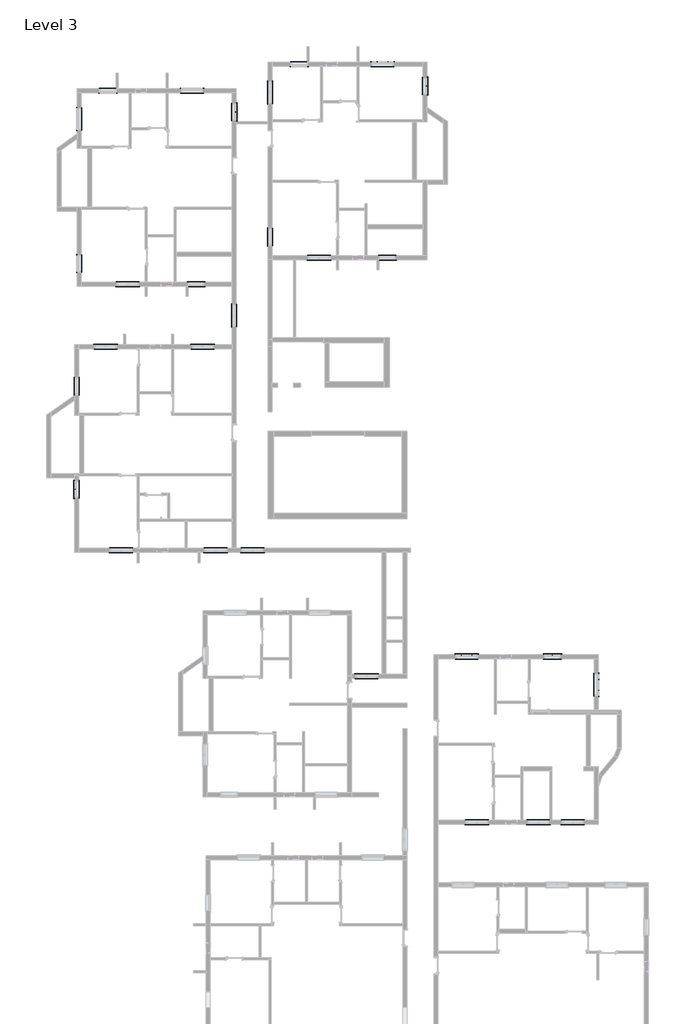
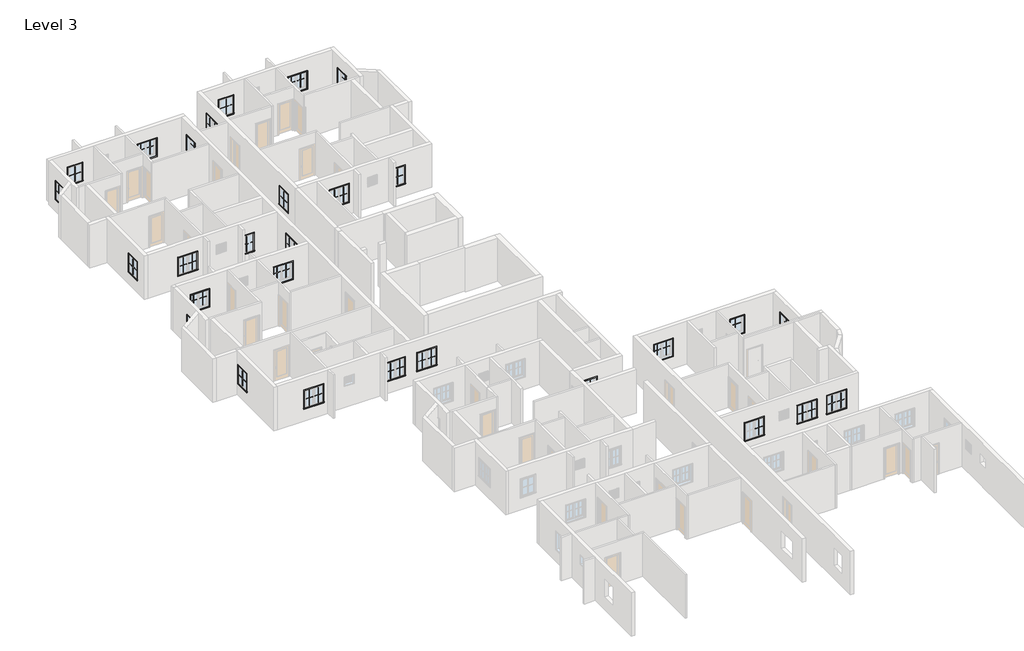
# One storey, part 7 of 7: 104 proxies.
"""IFC4 building model written with IfcOpenShell, lengths in millimetres."""

from ifc_helpers import new_model, si_unit, origin, place, context, project, spatial, transform, mapped, element, save
from components import muntin_pattern_2x2_muntin_pattern_2x2_95b57395, muntin_pattern_2x2_muntin_pattern_2x2_4dfeb3f3, muntin_pattern_2x2_muntin_pattern_2x2_e852a7e4, trim_window_exterior_flat_with_sill_e4b28ec3, trim_window_exterior_flat_with_sill_7cfdd449, trim_window_interior_flat_picture_frame_39ff4276, trim_window_interior_flat_picture_frame_f1e0b15b

model = new_model("IFC4")

# Units and contexts
model_context = context("Model", 3, world=origin())
ifc_project = project(units=[si_unit("LENGTHUNIT", "METRE", prefix="MILLI")], contexts=[model_context])

# Site, building, storey
site = spatial("IfcSite", under=ifc_project)
building = spatial("IfcBuilding", under=site)
storey = spatial("IfcBuildingStorey", under=building, Name="Level 3", Elevation=3200.4)

# Proxies
placement = place(None, origin())
muntin_pattern_2x2_muntin_pattern_2x2_shape = muntin_pattern_2x2_muntin_pattern_2x2_95b57395(model_context)
element("IfcBuildingElementProxy", 1, Name="Muntin Pattern_2x2 : Muntin Pattern_2x2", ObjectType="Muntin Pattern_2x2 : Muntin Pattern_2x2", at=placement, inside=storey, context=model_context, shape_type="MappedRepresentation", body=[
    mapped(muntin_pattern_2x2_muntin_pattern_2x2_shape, transform((-14884.6759469, 4921.5461172, 4184.65), x_axis=(0.0, 1.0, 0.0), y_axis=(-1.0, 0.0, 0.0), z_axis=(0.0, 0.0, 1.0))),
])
element("IfcBuildingElementProxy", 2, Name="Muntin Pattern_2x2 : Muntin Pattern_2x2", ObjectType="Muntin Pattern_2x2 : Muntin Pattern_2x2", at=placement, inside=storey, context=model_context, shape_type="MappedRepresentation", body=[
    mapped(muntin_pattern_2x2_muntin_pattern_2x2_shape, transform((-12990.7362554, 27537.0711172, 4184.65), x_axis=(-1.0, 0.0, 0.0), y_axis=(0.0, -1.0, 0.0), z_axis=(0.0, 0.0, 1.0))),
])
element("IfcBuildingElementProxy", 3, Name="Muntin Pattern_2x2 : Muntin Pattern_2x2", ObjectType="Muntin Pattern_2x2 : Muntin Pattern_2x2", at=placement, inside=storey, context=model_context, shape_type="MappedRepresentation", body=[
    mapped(muntin_pattern_2x2_muntin_pattern_2x2_shape, transform((-5683.5259469, 26431.1755084, 4184.65), x_axis=(0.0, -1.0, 0.0), y_axis=(1.0, 0.0, 0.0), z_axis=(0.0, 0.0, 1.0))),
])
element("IfcBuildingElementProxy", 4, Name="Muntin Pattern_2x2 : Muntin Pattern_2x2", ObjectType="Muntin Pattern_2x2 : Muntin Pattern_2x2", at=placement, inside=storey, context=model_context, shape_type="MappedRepresentation", body=[
    mapped(muntin_pattern_2x2_muntin_pattern_2x2_shape, transform((-7960.0009469, 16513.4711172, 4184.65), x_axis=(-1.0, 0.0, 0.0), y_axis=(0.0, -1.0, 0.0), z_axis=(0.0, 0.0, 1.0))),
])
element("IfcBuildingElementProxy", 5, Name="Muntin Pattern_2x2 : Muntin Pattern_2x2", ObjectType="Muntin Pattern_2x2 : Muntin Pattern_2x2", at=placement, inside=storey, context=model_context, shape_type="MappedRepresentation", body=[
    mapped(muntin_pattern_2x2_muntin_pattern_2x2_shape, transform((-14732.2759469, 17786.6461172, 4184.65), x_axis=(0.0, 1.0, 0.0), y_axis=(-1.0, 0.0, 0.0), z_axis=(0.0, 0.0, 1.0))),
])
element("IfcBuildingElementProxy", 6, Name="Muntin Pattern_2x2 : Muntin Pattern_2x2", ObjectType="Muntin Pattern_2x2 : Muntin Pattern_2x2", at=placement, inside=storey, context=model_context, shape_type="MappedRepresentation", body=[
    mapped(muntin_pattern_2x2_muntin_pattern_2x2_shape, transform((-2075.0862554, 29050.5505084, 4184.65), x_axis=(-1.0, 0.0, 0.0), y_axis=(0.0, -1.0, 0.0), z_axis=(0.0, 0.0, 1.0))),
])
element("IfcBuildingElementProxy", 7, Name="Muntin Pattern_2x2 : Muntin Pattern_2x2", ObjectType="Muntin Pattern_2x2 : Muntin Pattern_2x2", at=placement, inside=storey, context=model_context, shape_type="MappedRepresentation", body=[
    mapped(muntin_pattern_2x2_muntin_pattern_2x2_shape, transform((5213.0740531, 27910.7255084, 4184.65), x_axis=(0.0, -1.0, 0.0), y_axis=(1.0, 0.0, 0.0), z_axis=(0.0, 0.0, 1.0))),
])
element("IfcBuildingElementProxy", 8, Name="Muntin Pattern_2x2 : Muntin Pattern_2x2", ObjectType="Muntin Pattern_2x2 : Muntin Pattern_2x2", at=placement, inside=storey, context=model_context, shape_type="MappedRepresentation", body=[
    mapped(muntin_pattern_2x2_muntin_pattern_2x2_shape, transform((2936.5990531, 18026.9505084, 4184.65), x_axis=(-1.0, 0.0, 0.0), y_axis=(0.0, -1.0, 0.0), z_axis=(0.0, 0.0, 1.0))),
])
element("IfcBuildingElementProxy", 9, Name="Muntin Pattern_2x2 : Muntin Pattern_2x2", ObjectType="Muntin Pattern_2x2 : Muntin Pattern_2x2", at=placement, inside=storey, context=model_context, shape_type="MappedRepresentation", body=[
    mapped(muntin_pattern_2x2_muntin_pattern_2x2_shape, transform((-3835.6759469, 19300.1255084, 4184.65), x_axis=(0.0, 1.0, 0.0), y_axis=(-1.0, 0.0, 0.0), z_axis=(0.0, 0.0, 1.0))),
])
element("IfcBuildingElementProxy", 10, Name="Muntin Pattern_2x2 : Muntin Pattern_2x2", ObjectType="Muntin Pattern_2x2 : Muntin Pattern_2x2", at=placement, inside=storey, context=model_context, shape_type="MappedRepresentation", body=[
    mapped(muntin_pattern_2x2_muntin_pattern_2x2_shape, transform((12366.3490531, -4512.6747229, 4184.65), x_axis=(1.0, 0.0, 0.0), y_axis=(0.0, 1.0, 0.0), z_axis=(0.0, 0.0, 1.0))),
])
element("IfcBuildingElementProxy", 11, Name="Muntin Pattern_2x2 : Muntin Pattern_2x2", ObjectType="Muntin Pattern_2x2 : Muntin Pattern_2x2", at=placement, inside=storey, context=model_context, shape_type="MappedRepresentation", body=[
    mapped(muntin_pattern_2x2_muntin_pattern_2x2_shape, transform((-14675.1259469, 10795.2961172, 4184.65), x_axis=(0.0, -1.0, 0.0), y_axis=(1.0, 0.0, 0.0), z_axis=(0.0, 0.0, 1.0))),
])
muntin_pattern_2x2_muntin_pattern_2x2_2_shape = muntin_pattern_2x2_muntin_pattern_2x2_4dfeb3f3(model_context)
element("IfcBuildingElementProxy", 12, Name="Muntin Pattern_2x2 : Muntin Pattern_2x2", ObjectType="Muntin Pattern_2x2 : Muntin Pattern_2x2", at=placement, inside=storey, context=model_context, shape_type="MappedRepresentation", body=[
    mapped(muntin_pattern_2x2_muntin_pattern_2x2_2_shape, transform((-8498.1634469, 27746.6211172, 4184.65), x_axis=(1.0, 0.0, 0.0), y_axis=(0.0, 1.0, 0.0), z_axis=(0.0, 0.0, 1.0))),
])
element("IfcBuildingElementProxy", 13, Name="Muntin Pattern_2x2 : Muntin Pattern_2x2", ObjectType="Muntin Pattern_2x2 : Muntin Pattern_2x2", at=placement, inside=storey, context=model_context, shape_type="MappedRepresentation", body=[
    mapped(muntin_pattern_2x2_muntin_pattern_2x2_2_shape, transform((-14732.2759469, 25728.9086172, 4184.65), x_axis=(0.0, 1.0, 0.0), y_axis=(-1.0, 0.0, 0.0), z_axis=(0.0, 0.0, 1.0))),
])
element("IfcBuildingElementProxy", 14, Name="Muntin Pattern_2x2 : Muntin Pattern_2x2", ObjectType="Muntin Pattern_2x2 : Muntin Pattern_2x2", at=placement, inside=storey, context=model_context, shape_type="MappedRepresentation", body=[
    mapped(muntin_pattern_2x2_muntin_pattern_2x2_2_shape, transform((-11562.0384469, 16513.4711172, 4184.65), x_axis=(-1.0, 0.0, 0.0), y_axis=(0.0, -1.0, 0.0), z_axis=(0.0, 0.0, 1.0))),
])
element("IfcBuildingElementProxy", 15, Name="Muntin Pattern_2x2 : Muntin Pattern_2x2", ObjectType="Muntin Pattern_2x2 : Muntin Pattern_2x2", at=placement, inside=storey, context=model_context, shape_type="MappedRepresentation", body=[
    mapped(muntin_pattern_2x2_muntin_pattern_2x2_2_shape, transform((-3835.6759469, 27242.3880084, 4184.65), x_axis=(0.0, 1.0, 0.0), y_axis=(-1.0, 0.0, 0.0), z_axis=(0.0, 0.0, 1.0))),
])
element("IfcBuildingElementProxy", 16, Name="Muntin Pattern_2x2 : Muntin Pattern_2x2", ObjectType="Muntin Pattern_2x2 : Muntin Pattern_2x2", at=placement, inside=storey, context=model_context, shape_type="MappedRepresentation", body=[
    mapped(muntin_pattern_2x2_muntin_pattern_2x2_2_shape, transform((2373.0365531, 29260.1005084, 4184.65), x_axis=(1.0, 0.0, 0.0), y_axis=(0.0, 1.0, 0.0), z_axis=(0.0, 0.0, 1.0))),
])
element("IfcBuildingElementProxy", 17, Name="Muntin Pattern_2x2 : Muntin Pattern_2x2", ObjectType="Muntin Pattern_2x2 : Muntin Pattern_2x2", at=placement, inside=storey, context=model_context, shape_type="MappedRepresentation", body=[
    mapped(muntin_pattern_2x2_muntin_pattern_2x2_2_shape, transform((-640.0384469, 18026.9505084, 4184.65), x_axis=(-1.0, 0.0, 0.0), y_axis=(0.0, -1.0, 0.0), z_axis=(0.0, 0.0, 1.0))),
])
element("IfcBuildingElementProxy", 18, Name="Muntin Pattern_2x2 : Muntin Pattern_2x2", ObjectType="Muntin Pattern_2x2 : Muntin Pattern_2x2", at=placement, inside=storey, context=model_context, shape_type="MappedRepresentation", body=[
    mapped(muntin_pattern_2x2_muntin_pattern_2x2_2_shape, transform((14979.3740531, -5923.9622229, 4184.65), x_axis=(0.0, -1.0, 0.0), y_axis=(1.0, 0.0, 0.0), z_axis=(0.0, 0.0, 1.0))),
])
element("IfcBuildingElementProxy", 19, Name="Muntin Pattern_2x2 : Muntin Pattern_2x2", ObjectType="Muntin Pattern_2x2 : Muntin Pattern_2x2", at=placement, inside=storey, context=model_context, shape_type="MappedRepresentation", body=[
    mapped(muntin_pattern_2x2_muntin_pattern_2x2_2_shape, transform((7173.6365531, -4512.6747229, 4184.65), x_axis=(1.0, 0.0, 0.0), y_axis=(0.0, 1.0, 0.0), z_axis=(0.0, 0.0, 1.0))),
])
element("IfcBuildingElementProxy", 20, Name="Muntin Pattern_2x2 : Muntin Pattern_2x2", ObjectType="Muntin Pattern_2x2 : Muntin Pattern_2x2", at=placement, inside=storey, context=model_context, shape_type="MappedRepresentation", body=[
    mapped(muntin_pattern_2x2_muntin_pattern_2x2_2_shape, transform((13825.2615531, -14158.3247229, 4184.65), x_axis=(-1.0, 0.0, 0.0), y_axis=(0.0, -1.0, 0.0), z_axis=(0.0, 0.0, 1.0))),
])
element("IfcBuildingElementProxy", 21, Name="Muntin Pattern_2x2 : Muntin Pattern_2x2", ObjectType="Muntin Pattern_2x2 : Muntin Pattern_2x2", at=placement, inside=storey, context=model_context, shape_type="MappedRepresentation", body=[
    mapped(muntin_pattern_2x2_muntin_pattern_2x2_2_shape, transform((11869.4615531, -14158.3247229, 4184.65), x_axis=(-1.0, 0.0, 0.0), y_axis=(0.0, -1.0, 0.0), z_axis=(0.0, 0.0, 1.0))),
])
element("IfcBuildingElementProxy", 22, Name="Muntin Pattern_2x2 : Muntin Pattern_2x2", ObjectType="Muntin Pattern_2x2 : Muntin Pattern_2x2", at=placement, inside=storey, context=model_context, shape_type="MappedRepresentation", body=[
    mapped(muntin_pattern_2x2_muntin_pattern_2x2_2_shape, transform((8364.2615531, -14158.3247229, 4184.65), x_axis=(-1.0, 0.0, 0.0), y_axis=(0.0, -1.0, 0.0), z_axis=(0.0, 0.0, 1.0))),
])
element("IfcBuildingElementProxy", 23, Name="Muntin Pattern_2x2 : Muntin Pattern_2x2", ObjectType="Muntin Pattern_2x2 : Muntin Pattern_2x2", at=placement, inside=storey, context=model_context, shape_type="MappedRepresentation", body=[
    mapped(muntin_pattern_2x2_muntin_pattern_2x2_2_shape, transform((1464.9865531, -5641.6788828, 4184.65), x_axis=(1.0, 0.0, 0.0), y_axis=(0.0, 1.0, 0.0), z_axis=(0.0, 0.0, 1.0))),
])
element("IfcBuildingElementProxy", 24, Name="Muntin Pattern_2x2 : Muntin Pattern_2x2", ObjectType="Muntin Pattern_2x2 : Muntin Pattern_2x2", at=placement, inside=storey, context=model_context, shape_type="MappedRepresentation", body=[
    mapped(muntin_pattern_2x2_muntin_pattern_2x2_2_shape, transform((-4443.6884469, 1349.6711172, 4184.65), x_axis=(-1.0, 0.0, 0.0), y_axis=(0.0, -1.0, 0.0), z_axis=(0.0, 0.0, 1.0))),
])
element("IfcBuildingElementProxy", 25, Name="Muntin Pattern_2x2 : Muntin Pattern_2x2", ObjectType="Muntin Pattern_2x2 : Muntin Pattern_2x2", at=placement, inside=storey, context=model_context, shape_type="MappedRepresentation", body=[
    mapped(muntin_pattern_2x2_muntin_pattern_2x2_2_shape, transform((-6540.8708092, 1349.6711172, 4184.65), x_axis=(-1.0, 0.0, 0.0), y_axis=(0.0, -1.0, 0.0), z_axis=(0.0, 0.0, 1.0))),
])
element("IfcBuildingElementProxy", 26, Name="Muntin Pattern_2x2 : Muntin Pattern_2x2", ObjectType="Muntin Pattern_2x2 : Muntin Pattern_2x2", at=placement, inside=storey, context=model_context, shape_type="MappedRepresentation", body=[
    mapped(muntin_pattern_2x2_muntin_pattern_2x2_2_shape, transform((-11943.0384469, 1349.6711172, 4184.65), x_axis=(-1.0, 0.0, 0.0), y_axis=(0.0, -1.0, 0.0), z_axis=(0.0, 0.0, 1.0))),
])
element("IfcBuildingElementProxy", 27, Name="Muntin Pattern_2x2 : Muntin Pattern_2x2", ObjectType="Muntin Pattern_2x2 : Muntin Pattern_2x2", at=placement, inside=storey, context=model_context, shape_type="MappedRepresentation", body=[
    mapped(muntin_pattern_2x2_muntin_pattern_2x2_2_shape, transform((-13424.2323258, 13141.6211172, 4184.65), x_axis=(1.0, 0.0, 0.0), y_axis=(0.0, 1.0, 0.0), z_axis=(0.0, 0.0, 1.0))),
])
element("IfcBuildingElementProxy", 28, Name="Muntin Pattern_2x2 : Muntin Pattern_2x2", ObjectType="Muntin Pattern_2x2 : Muntin Pattern_2x2", at=placement, inside=storey, context=model_context, shape_type="MappedRepresentation", body=[
    mapped(muntin_pattern_2x2_muntin_pattern_2x2_2_shape, transform((-7888.5634469, 13141.6211172, 4184.65), x_axis=(1.0, 0.0, 0.0), y_axis=(0.0, 1.0, 0.0), z_axis=(0.0, 0.0, 1.0))),
])
element("IfcBuildingElementProxy", 29, Name="Muntin Pattern_2x2 : Muntin Pattern_2x2", ObjectType="Muntin Pattern_2x2 : Muntin Pattern_2x2", at=placement, inside=storey, context=model_context, shape_type="MappedRepresentation", body=[
    mapped(muntin_pattern_2x2_muntin_pattern_2x2_2_shape, transform((-5893.0759469, 14524.3336172, 4184.65), x_axis=(0.0, 1.0, 0.0), y_axis=(-1.0, 0.0, 0.0), z_axis=(0.0, 0.0, 1.0))),
])
muntin_pattern_2x2_muntin_pattern_2x2_3_shape = muntin_pattern_2x2_muntin_pattern_2x2_e852a7e4(model_context)
element("IfcBuildingElementProxy", 30, Name="Muntin Pattern_2x2 : Muntin Pattern_2x2", ObjectType="Muntin Pattern_2x2 : Muntin Pattern_2x2", at=placement, inside=storey, context=model_context, shape_type="MappedRepresentation", body=[
    mapped(muntin_pattern_2x2_muntin_pattern_2x2_3_shape, transform((-7891.7384469, 27746.6211172, 4184.65), x_axis=(-1.0, 0.0, 0.0), y_axis=(0.0, -1.0, 0.0), z_axis=(0.0, 0.0, 1.0))),
])
element("IfcBuildingElementProxy", 31, Name="Muntin Pattern_2x2 : Muntin Pattern_2x2", ObjectType="Muntin Pattern_2x2 : Muntin Pattern_2x2", at=placement, inside=storey, context=model_context, shape_type="MappedRepresentation", body=[
    mapped(muntin_pattern_2x2_muntin_pattern_2x2_3_shape, transform((-14732.2759469, 26335.3336172, 4184.65), x_axis=(0.0, -1.0, 0.0), y_axis=(1.0, 0.0, 0.0), z_axis=(0.0, 0.0, 1.0))),
])
element("IfcBuildingElementProxy", 32, Name="Muntin Pattern_2x2 : Muntin Pattern_2x2", ObjectType="Muntin Pattern_2x2 : Muntin Pattern_2x2", at=placement, inside=storey, context=model_context, shape_type="MappedRepresentation", body=[
    mapped(muntin_pattern_2x2_muntin_pattern_2x2_3_shape, transform((-12168.4634469, 16513.4711172, 4184.65), x_axis=(1.0, 0.0, 0.0), y_axis=(0.0, 1.0, 0.0), z_axis=(0.0, 0.0, 1.0))),
])
element("IfcBuildingElementProxy", 33, Name="Muntin Pattern_2x2 : Muntin Pattern_2x2", ObjectType="Muntin Pattern_2x2 : Muntin Pattern_2x2", at=placement, inside=storey, context=model_context, shape_type="MappedRepresentation", body=[
    mapped(muntin_pattern_2x2_muntin_pattern_2x2_3_shape, transform((-3835.6759469, 27848.8130084, 4184.65), x_axis=(0.0, -1.0, 0.0), y_axis=(1.0, 0.0, 0.0), z_axis=(0.0, 0.0, 1.0))),
])
element("IfcBuildingElementProxy", 34, Name="Muntin Pattern_2x2 : Muntin Pattern_2x2", ObjectType="Muntin Pattern_2x2 : Muntin Pattern_2x2", at=placement, inside=storey, context=model_context, shape_type="MappedRepresentation", body=[
    mapped(muntin_pattern_2x2_muntin_pattern_2x2_3_shape, transform((2979.4615531, 29260.1005084, 4184.65), x_axis=(-1.0, 0.0, 0.0), y_axis=(0.0, -1.0, 0.0), z_axis=(0.0, 0.0, 1.0))),
])
element("IfcBuildingElementProxy", 35, Name="Muntin Pattern_2x2 : Muntin Pattern_2x2", ObjectType="Muntin Pattern_2x2 : Muntin Pattern_2x2", at=placement, inside=storey, context=model_context, shape_type="MappedRepresentation", body=[
    mapped(muntin_pattern_2x2_muntin_pattern_2x2_3_shape, transform((-1246.4634469, 18026.9505084, 4184.65), x_axis=(1.0, 0.0, 0.0), y_axis=(0.0, 1.0, 0.0), z_axis=(0.0, 0.0, 1.0))),
])
element("IfcBuildingElementProxy", 36, Name="Muntin Pattern_2x2 : Muntin Pattern_2x2", ObjectType="Muntin Pattern_2x2 : Muntin Pattern_2x2", at=placement, inside=storey, context=model_context, shape_type="MappedRepresentation", body=[
    mapped(muntin_pattern_2x2_muntin_pattern_2x2_3_shape, transform((14979.3740531, -6530.3872229, 4184.65), x_axis=(0.0, 1.0, 0.0), y_axis=(-1.0, 0.0, 0.0), z_axis=(0.0, 0.0, 1.0))),
])
element("IfcBuildingElementProxy", 37, Name="Muntin Pattern_2x2 : Muntin Pattern_2x2", ObjectType="Muntin Pattern_2x2 : Muntin Pattern_2x2", at=placement, inside=storey, context=model_context, shape_type="MappedRepresentation", body=[
    mapped(muntin_pattern_2x2_muntin_pattern_2x2_3_shape, transform((7780.0615531, -4512.6747229, 4184.65), x_axis=(-1.0, 0.0, 0.0), y_axis=(0.0, -1.0, 0.0), z_axis=(0.0, 0.0, 1.0))),
])
element("IfcBuildingElementProxy", 38, Name="Muntin Pattern_2x2 : Muntin Pattern_2x2", ObjectType="Muntin Pattern_2x2 : Muntin Pattern_2x2", at=placement, inside=storey, context=model_context, shape_type="MappedRepresentation", body=[
    mapped(muntin_pattern_2x2_muntin_pattern_2x2_3_shape, transform((13218.8365531, -14158.3247229, 4184.65), x_axis=(1.0, 0.0, 0.0), y_axis=(0.0, 1.0, 0.0), z_axis=(0.0, 0.0, 1.0))),
])
element("IfcBuildingElementProxy", 39, Name="Muntin Pattern_2x2 : Muntin Pattern_2x2", ObjectType="Muntin Pattern_2x2 : Muntin Pattern_2x2", at=placement, inside=storey, context=model_context, shape_type="MappedRepresentation", body=[
    mapped(muntin_pattern_2x2_muntin_pattern_2x2_3_shape, transform((11263.0365531, -14158.3247229, 4184.65), x_axis=(1.0, 0.0, 0.0), y_axis=(0.0, 1.0, 0.0), z_axis=(0.0, 0.0, 1.0))),
])
element("IfcBuildingElementProxy", 40, Name="Muntin Pattern_2x2 : Muntin Pattern_2x2", ObjectType="Muntin Pattern_2x2 : Muntin Pattern_2x2", at=placement, inside=storey, context=model_context, shape_type="MappedRepresentation", body=[
    mapped(muntin_pattern_2x2_muntin_pattern_2x2_3_shape, transform((2071.4115531, -5641.6788828, 4184.65), x_axis=(-1.0, 0.0, 0.0), y_axis=(0.0, -1.0, 0.0), z_axis=(0.0, 0.0, 1.0))),
])
element("IfcBuildingElementProxy", 41, Name="Muntin Pattern_2x2 : Muntin Pattern_2x2", ObjectType="Muntin Pattern_2x2 : Muntin Pattern_2x2", at=placement, inside=storey, context=model_context, shape_type="MappedRepresentation", body=[
    mapped(muntin_pattern_2x2_muntin_pattern_2x2_3_shape, transform((-5050.1134469, 1349.6711172, 4184.65), x_axis=(1.0, 0.0, 0.0), y_axis=(0.0, 1.0, 0.0), z_axis=(0.0, 0.0, 1.0))),
])
element("IfcBuildingElementProxy", 42, Name="Muntin Pattern_2x2 : Muntin Pattern_2x2", ObjectType="Muntin Pattern_2x2 : Muntin Pattern_2x2", at=placement, inside=storey, context=model_context, shape_type="MappedRepresentation", body=[
    mapped(muntin_pattern_2x2_muntin_pattern_2x2_3_shape, transform((-7147.2958092, 1349.6711172, 4184.65), x_axis=(1.0, 0.0, 0.0), y_axis=(0.0, 1.0, 0.0), z_axis=(0.0, 0.0, 1.0))),
])
element("IfcBuildingElementProxy", 43, Name="Muntin Pattern_2x2 : Muntin Pattern_2x2", ObjectType="Muntin Pattern_2x2 : Muntin Pattern_2x2", at=placement, inside=storey, context=model_context, shape_type="MappedRepresentation", body=[
    mapped(muntin_pattern_2x2_muntin_pattern_2x2_3_shape, transform((-12549.4634469, 1349.6711172, 4184.65), x_axis=(1.0, 0.0, 0.0), y_axis=(0.0, 1.0, 0.0), z_axis=(0.0, 0.0, 1.0))),
])
element("IfcBuildingElementProxy", 44, Name="Muntin Pattern_2x2 : Muntin Pattern_2x2", ObjectType="Muntin Pattern_2x2 : Muntin Pattern_2x2", at=placement, inside=storey, context=model_context, shape_type="MappedRepresentation", body=[
    mapped(muntin_pattern_2x2_muntin_pattern_2x2_3_shape, transform((-12817.8073258, 13141.6211172, 4184.65), x_axis=(-1.0, 0.0, 0.0), y_axis=(0.0, -1.0, 0.0), z_axis=(0.0, 0.0, 1.0))),
])
element("IfcBuildingElementProxy", 45, Name="Muntin Pattern_2x2 : Muntin Pattern_2x2", ObjectType="Muntin Pattern_2x2 : Muntin Pattern_2x2", at=placement, inside=storey, context=model_context, shape_type="MappedRepresentation", body=[
    mapped(muntin_pattern_2x2_muntin_pattern_2x2_3_shape, transform((-7282.1384469, 13141.6211172, 4184.65), x_axis=(-1.0, 0.0, 0.0), y_axis=(0.0, -1.0, 0.0), z_axis=(0.0, 0.0, 1.0))),
])
element("IfcBuildingElementProxy", 46, Name="Muntin Pattern_2x2 : Muntin Pattern_2x2", ObjectType="Muntin Pattern_2x2 : Muntin Pattern_2x2", at=placement, inside=storey, context=model_context, shape_type="MappedRepresentation", body=[
    mapped(muntin_pattern_2x2_muntin_pattern_2x2_3_shape, transform((-5893.0759469, 15130.7586172, 4184.65), x_axis=(0.0, -1.0, 0.0), y_axis=(1.0, 0.0, 0.0), z_axis=(0.0, 0.0, 1.0))),
])
trim_window_exterior_flat_with_sill_shape = trim_window_exterior_flat_with_sill_e4b28ec3(model_context)
element("IfcBuildingElementProxy", 47, Name="Trim-Window-Exterior-Flat : with Sill", ObjectType="Trim-Window-Exterior-Flat : with Sill", at=placement, inside=storey, context=model_context, shape_type="MappedRepresentation", body=[
    mapped(trim_window_exterior_flat_with_sill_shape, transform((-14894.2009469, 4921.5461172, 5334.0), x_axis=(0.0, -1.0, 0.0), y_axis=(0.0, 0.0, 1.0), z_axis=(-1.0, 0.0, 0.0))),
])
element("IfcBuildingElementProxy", 48, Name="Trim-Window-Exterior-Flat : with Sill", ObjectType="Trim-Window-Exterior-Flat : with Sill", at=placement, inside=storey, context=model_context, shape_type="MappedRepresentation", body=[
    mapped(trim_window_exterior_flat_with_sill_shape, transform((-12990.7362554, 27527.5461172, 5334.0), x_axis=(1.0, 0.0, 0.0), y_axis=(0.0, 0.0, 1.0), z_axis=(0.0, -1.0, 0.0))),
])
element("IfcBuildingElementProxy", 49, Name="Trim-Window-Exterior-Flat : with Sill", ObjectType="Trim-Window-Exterior-Flat : with Sill", at=placement, inside=storey, context=model_context, shape_type="MappedRepresentation", body=[
    mapped(trim_window_exterior_flat_with_sill_shape, transform((-5674.0009469, 26431.1755084, 5334.0), x_axis=(0.0, 1.0, 0.0), y_axis=(0.0, 0.0, 1.0), z_axis=(1.0, 0.0, 0.0))),
])
element("IfcBuildingElementProxy", 50, Name="Trim-Window-Exterior-Flat : with Sill", ObjectType="Trim-Window-Exterior-Flat : with Sill", at=placement, inside=storey, context=model_context, shape_type="MappedRepresentation", body=[
    mapped(trim_window_exterior_flat_with_sill_shape, transform((-7960.0009469, 16503.9461172, 5334.0), x_axis=(1.0, 0.0, 0.0), y_axis=(0.0, 0.0, 1.0), z_axis=(0.0, -1.0, 0.0))),
])
element("IfcBuildingElementProxy", 51, Name="Trim-Window-Exterior-Flat : with Sill", ObjectType="Trim-Window-Exterior-Flat : with Sill", at=placement, inside=storey, context=model_context, shape_type="MappedRepresentation", body=[
    mapped(trim_window_exterior_flat_with_sill_shape, transform((-14741.8009469, 17786.6461172, 5334.0), x_axis=(0.0, -1.0, 0.0), y_axis=(0.0, 0.0, 1.0), z_axis=(-1.0, 0.0, 0.0))),
])
element("IfcBuildingElementProxy", 52, Name="Trim-Window-Exterior-Flat : with Sill", ObjectType="Trim-Window-Exterior-Flat : with Sill", at=placement, inside=storey, context=model_context, shape_type="MappedRepresentation", body=[
    mapped(trim_window_exterior_flat_with_sill_shape, transform((-2075.0862554, 29041.0255084, 5334.0), x_axis=(1.0, 0.0, 0.0), y_axis=(0.0, 0.0, 1.0), z_axis=(0.0, -1.0, 0.0))),
])
element("IfcBuildingElementProxy", 53, Name="Trim-Window-Exterior-Flat : with Sill", ObjectType="Trim-Window-Exterior-Flat : with Sill", at=placement, inside=storey, context=model_context, shape_type="MappedRepresentation", body=[
    mapped(trim_window_exterior_flat_with_sill_shape, transform((5222.5990531, 27910.7255084, 5334.0), x_axis=(0.0, 1.0, 0.0), y_axis=(0.0, 0.0, 1.0), z_axis=(1.0, 0.0, 0.0))),
])
element("IfcBuildingElementProxy", 54, Name="Trim-Window-Exterior-Flat : with Sill", ObjectType="Trim-Window-Exterior-Flat : with Sill", at=placement, inside=storey, context=model_context, shape_type="MappedRepresentation", body=[
    mapped(trim_window_exterior_flat_with_sill_shape, transform((2936.5990531, 18017.4255084, 5334.0), x_axis=(1.0, 0.0, 0.0), y_axis=(0.0, 0.0, 1.0), z_axis=(0.0, -1.0, 0.0))),
])
element("IfcBuildingElementProxy", 55, Name="Trim-Window-Exterior-Flat : with Sill", ObjectType="Trim-Window-Exterior-Flat : with Sill", at=placement, inside=storey, context=model_context, shape_type="MappedRepresentation", body=[
    mapped(trim_window_exterior_flat_with_sill_shape, transform((-3845.2009469, 19300.1255084, 5334.0), x_axis=(0.0, -1.0, 0.0), y_axis=(0.0, 0.0, 1.0), z_axis=(-1.0, 0.0, 0.0))),
])
element("IfcBuildingElementProxy", 56, Name="Trim-Window-Exterior-Flat : with Sill", ObjectType="Trim-Window-Exterior-Flat : with Sill", at=placement, inside=storey, context=model_context, shape_type="MappedRepresentation", body=[
    mapped(trim_window_exterior_flat_with_sill_shape, transform((12366.3490531, -4503.1497229, 5334.0), x_axis=(-1.0, 0.0, 0.0), y_axis=(0.0, 0.0, 1.0), z_axis=(0.0, 1.0, 0.0))),
])
element("IfcBuildingElementProxy", 57, Name="Trim-Window-Exterior-Flat : with Sill", ObjectType="Trim-Window-Exterior-Flat : with Sill", at=placement, inside=storey, context=model_context, shape_type="MappedRepresentation", body=[
    mapped(trim_window_exterior_flat_with_sill_shape, transform((-14665.6009469, 10795.2961172, 5334.0), x_axis=(0.0, 1.0, 0.0), y_axis=(0.0, 0.0, 1.0), z_axis=(1.0, 0.0, 0.0))),
])
trim_window_exterior_flat_with_sill_2_shape = trim_window_exterior_flat_with_sill_7cfdd449(model_context)
element("IfcBuildingElementProxy", 58, Name="Trim-Window-Exterior-Flat : with Sill", ObjectType="Trim-Window-Exterior-Flat : with Sill", at=placement, inside=storey, context=model_context, shape_type="MappedRepresentation", body=[
    mapped(trim_window_exterior_flat_with_sill_2_shape, transform((-8194.9509469, 27756.1461172, 5334.0), x_axis=(-1.0, 0.0, 0.0), y_axis=(0.0, 0.0, 1.0), z_axis=(0.0, 1.0, 0.0))),
])
element("IfcBuildingElementProxy", 59, Name="Trim-Window-Exterior-Flat : with Sill", ObjectType="Trim-Window-Exterior-Flat : with Sill", at=placement, inside=storey, context=model_context, shape_type="MappedRepresentation", body=[
    mapped(trim_window_exterior_flat_with_sill_2_shape, transform((-14741.8009469, 26032.1211172, 5334.0), x_axis=(0.0, -1.0, 0.0), y_axis=(0.0, 0.0, 1.0), z_axis=(-1.0, 0.0, 0.0))),
])
element("IfcBuildingElementProxy", 60, Name="Trim-Window-Exterior-Flat : with Sill", ObjectType="Trim-Window-Exterior-Flat : with Sill", at=placement, inside=storey, context=model_context, shape_type="MappedRepresentation", body=[
    mapped(trim_window_exterior_flat_with_sill_2_shape, transform((-11865.2509469, 16503.9461172, 5334.0), x_axis=(1.0, 0.0, 0.0), y_axis=(0.0, 0.0, 1.0), z_axis=(0.0, -1.0, 0.0))),
])
element("IfcBuildingElementProxy", 61, Name="Trim-Window-Exterior-Flat : with Sill", ObjectType="Trim-Window-Exterior-Flat : with Sill", at=placement, inside=storey, context=model_context, shape_type="MappedRepresentation", body=[
    mapped(trim_window_exterior_flat_with_sill_2_shape, transform((-3845.2009469, 27545.6005084, 5334.0), x_axis=(0.0, -1.0, 0.0), y_axis=(0.0, 0.0, 1.0), z_axis=(-1.0, 0.0, 0.0))),
])
element("IfcBuildingElementProxy", 62, Name="Trim-Window-Exterior-Flat : with Sill", ObjectType="Trim-Window-Exterior-Flat : with Sill", at=placement, inside=storey, context=model_context, shape_type="MappedRepresentation", body=[
    mapped(trim_window_exterior_flat_with_sill_2_shape, transform((2676.2490531, 29269.6255084, 5334.0), x_axis=(-1.0, 0.0, 0.0), y_axis=(0.0, 0.0, 1.0), z_axis=(0.0, 1.0, 0.0))),
])
element("IfcBuildingElementProxy", 63, Name="Trim-Window-Exterior-Flat : with Sill", ObjectType="Trim-Window-Exterior-Flat : with Sill", at=placement, inside=storey, context=model_context, shape_type="MappedRepresentation", body=[
    mapped(trim_window_exterior_flat_with_sill_2_shape, transform((-943.2509469, 18017.4255084, 5334.0), x_axis=(1.0, 0.0, 0.0), y_axis=(0.0, 0.0, 1.0), z_axis=(0.0, -1.0, 0.0))),
])
element("IfcBuildingElementProxy", 64, Name="Trim-Window-Exterior-Flat : with Sill", ObjectType="Trim-Window-Exterior-Flat : with Sill", at=placement, inside=storey, context=model_context, shape_type="MappedRepresentation", body=[
    mapped(trim_window_exterior_flat_with_sill_2_shape, transform((14988.8990531, -6227.1747229, 5334.0), x_axis=(0.0, 1.0, 0.0), y_axis=(0.0, 0.0, 1.0), z_axis=(1.0, 0.0, 0.0))),
])
element("IfcBuildingElementProxy", 65, Name="Trim-Window-Exterior-Flat : with Sill", ObjectType="Trim-Window-Exterior-Flat : with Sill", at=placement, inside=storey, context=model_context, shape_type="MappedRepresentation", body=[
    mapped(trim_window_exterior_flat_with_sill_2_shape, transform((7476.8490531, -4503.1497229, 5334.0), x_axis=(-1.0, 0.0, 0.0), y_axis=(0.0, 0.0, 1.0), z_axis=(0.0, 1.0, 0.0))),
])
element("IfcBuildingElementProxy", 66, Name="Trim-Window-Exterior-Flat : with Sill", ObjectType="Trim-Window-Exterior-Flat : with Sill", at=placement, inside=storey, context=model_context, shape_type="MappedRepresentation", body=[
    mapped(trim_window_exterior_flat_with_sill_2_shape, transform((13522.0490531, -14167.8497229, 5334.0), x_axis=(1.0, 0.0, 0.0), y_axis=(0.0, 0.0, 1.0), z_axis=(0.0, -1.0, 0.0))),
])
element("IfcBuildingElementProxy", 67, Name="Trim-Window-Exterior-Flat : with Sill", ObjectType="Trim-Window-Exterior-Flat : with Sill", at=placement, inside=storey, context=model_context, shape_type="MappedRepresentation", body=[
    mapped(trim_window_exterior_flat_with_sill_2_shape, transform((11566.2490531, -14167.8497229, 5334.0), x_axis=(1.0, 0.0, 0.0), y_axis=(0.0, 0.0, 1.0), z_axis=(0.0, -1.0, 0.0))),
])
element("IfcBuildingElementProxy", 68, Name="Trim-Window-Exterior-Flat : with Sill", ObjectType="Trim-Window-Exterior-Flat : with Sill", at=placement, inside=storey, context=model_context, shape_type="MappedRepresentation", body=[
    mapped(trim_window_exterior_flat_with_sill_2_shape, transform((8061.0490531, -14167.8497229, 5334.0), x_axis=(1.0, 0.0, 0.0), y_axis=(0.0, 0.0, 1.0), z_axis=(0.0, -1.0, 0.0))),
])
element("IfcBuildingElementProxy", 69, Name="Trim-Window-Exterior-Flat : with Sill", ObjectType="Trim-Window-Exterior-Flat : with Sill", at=placement, inside=storey, context=model_context, shape_type="MappedRepresentation", body=[
    mapped(trim_window_exterior_flat_with_sill_2_shape, transform((1768.1990531, -5632.1538828, 5334.0), x_axis=(-1.0, 0.0, 0.0), y_axis=(0.0, 0.0, 1.0), z_axis=(0.0, 1.0, 0.0))),
])
element("IfcBuildingElementProxy", 70, Name="Trim-Window-Exterior-Flat : with Sill", ObjectType="Trim-Window-Exterior-Flat : with Sill", at=placement, inside=storey, context=model_context, shape_type="MappedRepresentation", body=[
    mapped(trim_window_exterior_flat_with_sill_2_shape, transform((-4746.9009469, 1340.1461172, 5334.0), x_axis=(1.0, 0.0, 0.0), y_axis=(0.0, 0.0, 1.0), z_axis=(0.0, -1.0, 0.0))),
])
element("IfcBuildingElementProxy", 71, Name="Trim-Window-Exterior-Flat : with Sill", ObjectType="Trim-Window-Exterior-Flat : with Sill", at=placement, inside=storey, context=model_context, shape_type="MappedRepresentation", body=[
    mapped(trim_window_exterior_flat_with_sill_2_shape, transform((-6844.0833092, 1340.1461172, 5334.0), x_axis=(1.0, 0.0, 0.0), y_axis=(0.0, 0.0, 1.0), z_axis=(0.0, -1.0, 0.0))),
])
element("IfcBuildingElementProxy", 72, Name="Trim-Window-Exterior-Flat : with Sill", ObjectType="Trim-Window-Exterior-Flat : with Sill", at=placement, inside=storey, context=model_context, shape_type="MappedRepresentation", body=[
    mapped(trim_window_exterior_flat_with_sill_2_shape, transform((-12246.2509469, 1340.1461172, 5334.0), x_axis=(1.0, 0.0, 0.0), y_axis=(0.0, 0.0, 1.0), z_axis=(0.0, -1.0, 0.0))),
])
element("IfcBuildingElementProxy", 73, Name="Trim-Window-Exterior-Flat : with Sill", ObjectType="Trim-Window-Exterior-Flat : with Sill", at=placement, inside=storey, context=model_context, shape_type="MappedRepresentation", body=[
    mapped(trim_window_exterior_flat_with_sill_2_shape, transform((-13121.0198258, 13151.1461172, 5334.0), x_axis=(-1.0, 0.0, 0.0), y_axis=(0.0, 0.0, 1.0), z_axis=(0.0, 1.0, 0.0))),
])
element("IfcBuildingElementProxy", 74, Name="Trim-Window-Exterior-Flat : with Sill", ObjectType="Trim-Window-Exterior-Flat : with Sill", at=placement, inside=storey, context=model_context, shape_type="MappedRepresentation", body=[
    mapped(trim_window_exterior_flat_with_sill_2_shape, transform((-7585.3509469, 13151.1461172, 5334.0), x_axis=(-1.0, 0.0, 0.0), y_axis=(0.0, 0.0, 1.0), z_axis=(0.0, 1.0, 0.0))),
])
element("IfcBuildingElementProxy", 75, Name="Trim-Window-Exterior-Flat : with Sill", ObjectType="Trim-Window-Exterior-Flat : with Sill", at=placement, inside=storey, context=model_context, shape_type="MappedRepresentation", body=[
    mapped(trim_window_exterior_flat_with_sill_2_shape, transform((-5902.6009469, 14827.5461172, 5334.0), x_axis=(0.0, -1.0, 0.0), y_axis=(0.0, 0.0, 1.0), z_axis=(-1.0, 0.0, 0.0))),
])
trim_window_interior_flat_picture_frame_shape = trim_window_interior_flat_picture_frame_39ff4276(model_context)
element("IfcBuildingElementProxy", 76, Name="Trim-Window-Interior-Flat : Picture Frame", ObjectType="Trim-Window-Interior-Flat : Picture Frame", at=placement, inside=storey, context=model_context, shape_type="MappedRepresentation", body=[
    mapped(trim_window_interior_flat_picture_frame_shape, transform((-14665.6009469, 4921.5461172, 5334.0), x_axis=(0.0, 1.0, 0.0), y_axis=(0.0, 0.0, 1.0), z_axis=(1.0, 0.0, 0.0))),
])
element("IfcBuildingElementProxy", 77, Name="Trim-Window-Interior-Flat : Picture Frame", ObjectType="Trim-Window-Interior-Flat : Picture Frame", at=placement, inside=storey, context=model_context, shape_type="MappedRepresentation", body=[
    mapped(trim_window_interior_flat_picture_frame_shape, transform((-12990.7362554, 27756.1461172, 5334.0), x_axis=(-1.0, 0.0, 0.0), y_axis=(0.0, 0.0, 1.0), z_axis=(0.0, 1.0, 0.0))),
])
element("IfcBuildingElementProxy", 78, Name="Trim-Window-Interior-Flat : Picture Frame", ObjectType="Trim-Window-Interior-Flat : Picture Frame", at=placement, inside=storey, context=model_context, shape_type="MappedRepresentation", body=[
    mapped(trim_window_interior_flat_picture_frame_shape, transform((-5902.6009469, 26431.1755084, 5334.0), x_axis=(0.0, -1.0, 0.0), y_axis=(0.0, 0.0, 1.0), z_axis=(-1.0, 0.0, 0.0))),
])
element("IfcBuildingElementProxy", 79, Name="Trim-Window-Interior-Flat : Picture Frame", ObjectType="Trim-Window-Interior-Flat : Picture Frame", at=placement, inside=storey, context=model_context, shape_type="MappedRepresentation", body=[
    mapped(trim_window_interior_flat_picture_frame_shape, transform((-7960.0009469, 16732.5461172, 5334.0), x_axis=(-1.0, 0.0, 0.0), y_axis=(0.0, 0.0, 1.0), z_axis=(0.0, 1.0, 0.0))),
])
element("IfcBuildingElementProxy", 80, Name="Trim-Window-Interior-Flat : Picture Frame", ObjectType="Trim-Window-Interior-Flat : Picture Frame", at=placement, inside=storey, context=model_context, shape_type="MappedRepresentation", body=[
    mapped(trim_window_interior_flat_picture_frame_shape, transform((-14513.2009469, 17786.6461172, 5334.0), x_axis=(0.0, 1.0, 0.0), y_axis=(0.0, 0.0, 1.0), z_axis=(1.0, 0.0, 0.0))),
])
element("IfcBuildingElementProxy", 81, Name="Trim-Window-Interior-Flat : Picture Frame", ObjectType="Trim-Window-Interior-Flat : Picture Frame", at=placement, inside=storey, context=model_context, shape_type="MappedRepresentation", body=[
    mapped(trim_window_interior_flat_picture_frame_shape, transform((-2075.0862554, 29269.6255084, 5334.0), x_axis=(-1.0, 0.0, 0.0), y_axis=(0.0, 0.0, 1.0), z_axis=(0.0, 1.0, 0.0))),
])
element("IfcBuildingElementProxy", 82, Name="Trim-Window-Interior-Flat : Picture Frame", ObjectType="Trim-Window-Interior-Flat : Picture Frame", at=placement, inside=storey, context=model_context, shape_type="MappedRepresentation", body=[
    mapped(trim_window_interior_flat_picture_frame_shape, transform((4993.9990531, 27910.7255084, 5334.0), x_axis=(0.0, -1.0, 0.0), y_axis=(0.0, 0.0, 1.0), z_axis=(-1.0, 0.0, 0.0))),
])
element("IfcBuildingElementProxy", 83, Name="Trim-Window-Interior-Flat : Picture Frame", ObjectType="Trim-Window-Interior-Flat : Picture Frame", at=placement, inside=storey, context=model_context, shape_type="MappedRepresentation", body=[
    mapped(trim_window_interior_flat_picture_frame_shape, transform((2936.5990531, 18246.0255084, 5334.0), x_axis=(-1.0, 0.0, 0.0), y_axis=(0.0, 0.0, 1.0), z_axis=(0.0, 1.0, 0.0))),
])
element("IfcBuildingElementProxy", 84, Name="Trim-Window-Interior-Flat : Picture Frame", ObjectType="Trim-Window-Interior-Flat : Picture Frame", at=placement, inside=storey, context=model_context, shape_type="MappedRepresentation", body=[
    mapped(trim_window_interior_flat_picture_frame_shape, transform((-3616.6009469, 19300.1255084, 5334.0), x_axis=(0.0, 1.0, 0.0), y_axis=(0.0, 0.0, 1.0), z_axis=(1.0, 0.0, 0.0))),
])
element("IfcBuildingElementProxy", 85, Name="Trim-Window-Interior-Flat : Picture Frame", ObjectType="Trim-Window-Interior-Flat : Picture Frame", at=placement, inside=storey, context=model_context, shape_type="MappedRepresentation", body=[
    mapped(trim_window_interior_flat_picture_frame_shape, transform((12366.3490531, -4731.7497229, 5334.0), x_axis=(1.0, 0.0, 0.0), y_axis=(0.0, 0.0, 1.0), z_axis=(0.0, -1.0, 0.0))),
])
element("IfcBuildingElementProxy", 86, Name="Trim-Window-Interior-Flat : Picture Frame", ObjectType="Trim-Window-Interior-Flat : Picture Frame", at=placement, inside=storey, context=model_context, shape_type="MappedRepresentation", body=[
    mapped(trim_window_interior_flat_picture_frame_shape, transform((-14894.2009469, 10795.2961172, 5334.0), x_axis=(0.0, -1.0, 0.0), y_axis=(0.0, 0.0, 1.0), z_axis=(-1.0, 0.0, 0.0))),
])
trim_window_interior_flat_picture_frame_2_shape = trim_window_interior_flat_picture_frame_f1e0b15b(model_context)
element("IfcBuildingElementProxy", 87, Name="Trim-Window-Interior-Flat : Picture Frame", ObjectType="Trim-Window-Interior-Flat : Picture Frame", at=placement, inside=storey, context=model_context, shape_type="MappedRepresentation", body=[
    mapped(trim_window_interior_flat_picture_frame_2_shape, transform((-8194.9509469, 27527.5461172, 5334.0), x_axis=(1.0, 0.0, 0.0), y_axis=(0.0, 0.0, 1.0), z_axis=(0.0, -1.0, 0.0))),
])
element("IfcBuildingElementProxy", 88, Name="Trim-Window-Interior-Flat : Picture Frame", ObjectType="Trim-Window-Interior-Flat : Picture Frame", at=placement, inside=storey, context=model_context, shape_type="MappedRepresentation", body=[
    mapped(trim_window_interior_flat_picture_frame_2_shape, transform((-14513.2009469, 26032.1211172, 5334.0), x_axis=(0.0, 1.0, 0.0), y_axis=(0.0, 0.0, 1.0), z_axis=(1.0, 0.0, 0.0))),
])
element("IfcBuildingElementProxy", 89, Name="Trim-Window-Interior-Flat : Picture Frame", ObjectType="Trim-Window-Interior-Flat : Picture Frame", at=placement, inside=storey, context=model_context, shape_type="MappedRepresentation", body=[
    mapped(trim_window_interior_flat_picture_frame_2_shape, transform((-11865.2509469, 16732.5461172, 5334.0), x_axis=(-1.0, 0.0, 0.0), y_axis=(0.0, 0.0, 1.0), z_axis=(0.0, 1.0, 0.0))),
])
element("IfcBuildingElementProxy", 90, Name="Trim-Window-Interior-Flat : Picture Frame", ObjectType="Trim-Window-Interior-Flat : Picture Frame", at=placement, inside=storey, context=model_context, shape_type="MappedRepresentation", body=[
    mapped(trim_window_interior_flat_picture_frame_2_shape, transform((-3616.6009469, 27545.6005084, 5334.0), x_axis=(0.0, 1.0, 0.0), y_axis=(0.0, 0.0, 1.0), z_axis=(1.0, 0.0, 0.0))),
])
element("IfcBuildingElementProxy", 91, Name="Trim-Window-Interior-Flat : Picture Frame", ObjectType="Trim-Window-Interior-Flat : Picture Frame", at=placement, inside=storey, context=model_context, shape_type="MappedRepresentation", body=[
    mapped(trim_window_interior_flat_picture_frame_2_shape, transform((2676.2490531, 29041.0255084, 5334.0), x_axis=(1.0, 0.0, 0.0), y_axis=(0.0, 0.0, 1.0), z_axis=(0.0, -1.0, 0.0))),
])
element("IfcBuildingElementProxy", 92, Name="Trim-Window-Interior-Flat : Picture Frame", ObjectType="Trim-Window-Interior-Flat : Picture Frame", at=placement, inside=storey, context=model_context, shape_type="MappedRepresentation", body=[
    mapped(trim_window_interior_flat_picture_frame_2_shape, transform((-943.2509469, 18246.0255084, 5334.0), x_axis=(-1.0, 0.0, 0.0), y_axis=(0.0, 0.0, 1.0), z_axis=(0.0, 1.0, 0.0))),
])
element("IfcBuildingElementProxy", 93, Name="Trim-Window-Interior-Flat : Picture Frame", ObjectType="Trim-Window-Interior-Flat : Picture Frame", at=placement, inside=storey, context=model_context, shape_type="MappedRepresentation", body=[
    mapped(trim_window_interior_flat_picture_frame_2_shape, transform((14760.2990531, -6227.1747229, 5334.0), x_axis=(0.0, -1.0, 0.0), y_axis=(0.0, 0.0, 1.0), z_axis=(-1.0, 0.0, 0.0))),
])
element("IfcBuildingElementProxy", 94, Name="Trim-Window-Interior-Flat : Picture Frame", ObjectType="Trim-Window-Interior-Flat : Picture Frame", at=placement, inside=storey, context=model_context, shape_type="MappedRepresentation", body=[
    mapped(trim_window_interior_flat_picture_frame_2_shape, transform((7476.8490531, -4731.7497229, 5334.0), x_axis=(1.0, 0.0, 0.0), y_axis=(0.0, 0.0, 1.0), z_axis=(0.0, -1.0, 0.0))),
])
element("IfcBuildingElementProxy", 95, Name="Trim-Window-Interior-Flat : Picture Frame", ObjectType="Trim-Window-Interior-Flat : Picture Frame", at=placement, inside=storey, context=model_context, shape_type="MappedRepresentation", body=[
    mapped(trim_window_interior_flat_picture_frame_2_shape, transform((13522.0490531, -13939.2497229, 5334.0), x_axis=(-1.0, 0.0, 0.0), y_axis=(0.0, 0.0, 1.0), z_axis=(0.0, 1.0, 0.0))),
])
element("IfcBuildingElementProxy", 96, Name="Trim-Window-Interior-Flat : Picture Frame", ObjectType="Trim-Window-Interior-Flat : Picture Frame", at=placement, inside=storey, context=model_context, shape_type="MappedRepresentation", body=[
    mapped(trim_window_interior_flat_picture_frame_2_shape, transform((11566.2490531, -13939.2497229, 5334.0), x_axis=(-1.0, 0.0, 0.0), y_axis=(0.0, 0.0, 1.0), z_axis=(0.0, 1.0, 0.0))),
])
element("IfcBuildingElementProxy", 97, Name="Trim-Window-Interior-Flat : Picture Frame", ObjectType="Trim-Window-Interior-Flat : Picture Frame", at=placement, inside=storey, context=model_context, shape_type="MappedRepresentation", body=[
    mapped(trim_window_interior_flat_picture_frame_2_shape, transform((8061.0490531, -13939.2497229, 5334.0), x_axis=(-1.0, 0.0, 0.0), y_axis=(0.0, 0.0, 1.0), z_axis=(0.0, 1.0, 0.0))),
])
element("IfcBuildingElementProxy", 98, Name="Trim-Window-Interior-Flat : Picture Frame", ObjectType="Trim-Window-Interior-Flat : Picture Frame", at=placement, inside=storey, context=model_context, shape_type="MappedRepresentation", body=[
    mapped(trim_window_interior_flat_picture_frame_2_shape, transform((1768.1990531, -5860.7538828, 5334.0), x_axis=(1.0, 0.0, 0.0), y_axis=(0.0, 0.0, 1.0), z_axis=(0.0, -1.0, 0.0))),
])
element("IfcBuildingElementProxy", 99, Name="Trim-Window-Interior-Flat : Picture Frame", ObjectType="Trim-Window-Interior-Flat : Picture Frame", at=placement, inside=storey, context=model_context, shape_type="MappedRepresentation", body=[
    mapped(trim_window_interior_flat_picture_frame_2_shape, transform((-4746.9009469, 1568.7461172, 5334.0), x_axis=(-1.0, 0.0, 0.0), y_axis=(0.0, 0.0, 1.0), z_axis=(0.0, 1.0, 0.0))),
])
element("IfcBuildingElementProxy", 100, Name="Trim-Window-Interior-Flat : Picture Frame", ObjectType="Trim-Window-Interior-Flat : Picture Frame", at=placement, inside=storey, context=model_context, shape_type="MappedRepresentation", body=[
    mapped(trim_window_interior_flat_picture_frame_2_shape, transform((-6844.0833092, 1568.7461172, 5334.0), x_axis=(-1.0, 0.0, 0.0), y_axis=(0.0, 0.0, 1.0), z_axis=(0.0, 1.0, 0.0))),
])
element("IfcBuildingElementProxy", 101, Name="Trim-Window-Interior-Flat : Picture Frame", ObjectType="Trim-Window-Interior-Flat : Picture Frame", at=placement, inside=storey, context=model_context, shape_type="MappedRepresentation", body=[
    mapped(trim_window_interior_flat_picture_frame_2_shape, transform((-12246.2509469, 1568.7461172, 5334.0), x_axis=(-1.0, 0.0, 0.0), y_axis=(0.0, 0.0, 1.0), z_axis=(0.0, 1.0, 0.0))),
])
element("IfcBuildingElementProxy", 102, Name="Trim-Window-Interior-Flat : Picture Frame", ObjectType="Trim-Window-Interior-Flat : Picture Frame", at=placement, inside=storey, context=model_context, shape_type="MappedRepresentation", body=[
    mapped(trim_window_interior_flat_picture_frame_2_shape, transform((-13121.0198258, 12922.5461172, 5334.0), x_axis=(1.0, 0.0, 0.0), y_axis=(0.0, 0.0, 1.0), z_axis=(0.0, -1.0, 0.0))),
])
element("IfcBuildingElementProxy", 103, Name="Trim-Window-Interior-Flat : Picture Frame", ObjectType="Trim-Window-Interior-Flat : Picture Frame", at=placement, inside=storey, context=model_context, shape_type="MappedRepresentation", body=[
    mapped(trim_window_interior_flat_picture_frame_2_shape, transform((-7585.3509469, 12922.5461172, 5334.0), x_axis=(1.0, 0.0, 0.0), y_axis=(0.0, 0.0, 1.0), z_axis=(0.0, -1.0, 0.0))),
])
element("IfcBuildingElementProxy", 104, Name="Trim-Window-Interior-Flat : Picture Frame", ObjectType="Trim-Window-Interior-Flat : Picture Frame", at=placement, inside=storey, context=model_context, shape_type="MappedRepresentation", body=[
    mapped(trim_window_interior_flat_picture_frame_2_shape, transform((-5674.0009469, 14827.5461172, 5334.0), x_axis=(0.0, 1.0, 0.0), y_axis=(0.0, 0.0, 1.0), z_axis=(1.0, 0.0, 0.0))),
])

save(model, "model.ifc")

# Revit data of these elements
# Type "Muntin Pattern_2x2 : Muntin Pattern_2x2"
#   Width [instance default] = 4' - 0"
#   Thickness = 0' - 0 1/2"
#   Height [instance default] = 4' - 0"
#   Distance = 0' - 0 3/4"
#   Interior Material [instance default] = none
#   Exterior Material [instance default] = none
#   Default Elevation = 0
# Type "Trim-Window-Exterior-Flat : with Sill"
#   Trim Width = 0' - 2 1/4"
#   Trim Thickness_Picture Frame = 0' - 1 1/4"
#   Trim Thickness_with Sill = 0' - 0 3/4"
#   Sill Thickness = 0' - 1 1/4"
#   Opening Width [instance default] = 2' - 0"
#   Opening Height [instance default] = 3' - 0"
#   Default Elevation = 4' - 0"
#   Sill = yes
#   Picture Frame = no
#   Trim Material [instance default] = none
# Type "Trim-Window-Interior-Flat : Picture Frame"
#   Trim Thickness_Picture Frame = 0' - 1 1/4"
#   Trim Width = 0' - 2 1/4"
#   Trim Thickness_with Sill = 0' - 0 3/4"
#   Sill Thickness = 0' - 1 1/4"
#   Opening Width [instance default] = 2' - 0"
#   Opening Height [instance default] = 3' - 0"
#   Default Elevation = 4' - 0"
#   Sill = no
#   Picture Frame = yes
#   Trim Material [instance default] = none
# Elements 1, 2, 3, 4, 5, 6, 7, 8, 9, 10, 11 (IfcBuildingElementProxy, "Muntin Pattern_2x2 : Muntin Pattern_2x2")
#   Width = 2' - 6 1/2"
#   Height = 3' - 6 1/2"
#   Interior Material = Wood - Stained
#   Exterior Material = Clad - White
#   Phase Created = New Construction
#   Materials on its faces: "Clad - White", "Wood - Stained"
# Elements 12, 13, 14, 15, 16, 17, 18, 19, 20, 21, 22, 23, 24, 25, 26, 27, 28, 29, 30, 31, 32, 33, 34, 35, 36, 37, 38, 39, 40, 41, 42, 43, 44, 45, 46 (IfcBuildingElementProxy, "Muntin Pattern_2x2 : Muntin Pattern_2x2")
#   Width = 1' - 6 5/8"
#   Height = 3' - 6 1/2"
#   Interior Material = Wood - Stained
#   Exterior Material = Clad - White
#   Phase Created = New Construction
#   Materials on its faces: "Clad - White", "Wood - Stained"
# Elements 47, 48, 49, 50, 51, 52, 53, 54, 55, 56, 57 (IfcBuildingElementProxy, "Trim-Window-Exterior-Flat : with Sill")
#   Opening Width = 3' - 0"
#   Opening Height = 4' - 0"
#   Trim Material = Clad - White
#   Phase Created = New Construction
#   Materials on its faces: "Clad - White"
# Elements 58, 59, 60, 61, 62, 63, 64, 65, 66, 67, 68, 69, 70, 71, 72, 73, 74, 75 (IfcBuildingElementProxy, "Trim-Window-Exterior-Flat : with Sill")
#   Opening Width = 4' - 0"
#   Opening Height = 4' - 0"
#   Trim Material = Clad - White
#   Phase Created = New Construction
#   Materials on its faces: "Clad - White"
# Elements 76, 77, 78, 79, 80, 81, 82, 83, 84, 85, 86 (IfcBuildingElementProxy, "Trim-Window-Interior-Flat : Picture Frame")
#   Opening Width = 3' - 0"
#   Opening Height = 4' - 0"
#   Trim Material = Wood - Stained
#   Phase Created = New Construction
#   Materials on its faces: "Wood - Stained"
# Elements 87, 88, 89, 90, 91, 92, 93, 94, 95, 96, 97, 98, 99, 100, 101, 102, 103, 104 (IfcBuildingElementProxy, "Trim-Window-Interior-Flat : Picture Frame")
#   Opening Width = 4' - 0"
#   Opening Height = 4' - 0"
#   Trim Material = Wood - Stained
#   Phase Created = New Construction
#   Materials on its faces: "Wood - Stained"
# Materials
#   "Clad - White": class "Wood", colour RGB 242 242 238, transparency 0, Cost = 0
#   "Wood - Stained": class "Wood", colour RGB 224 178 126, transparency 0, Cost = 0
